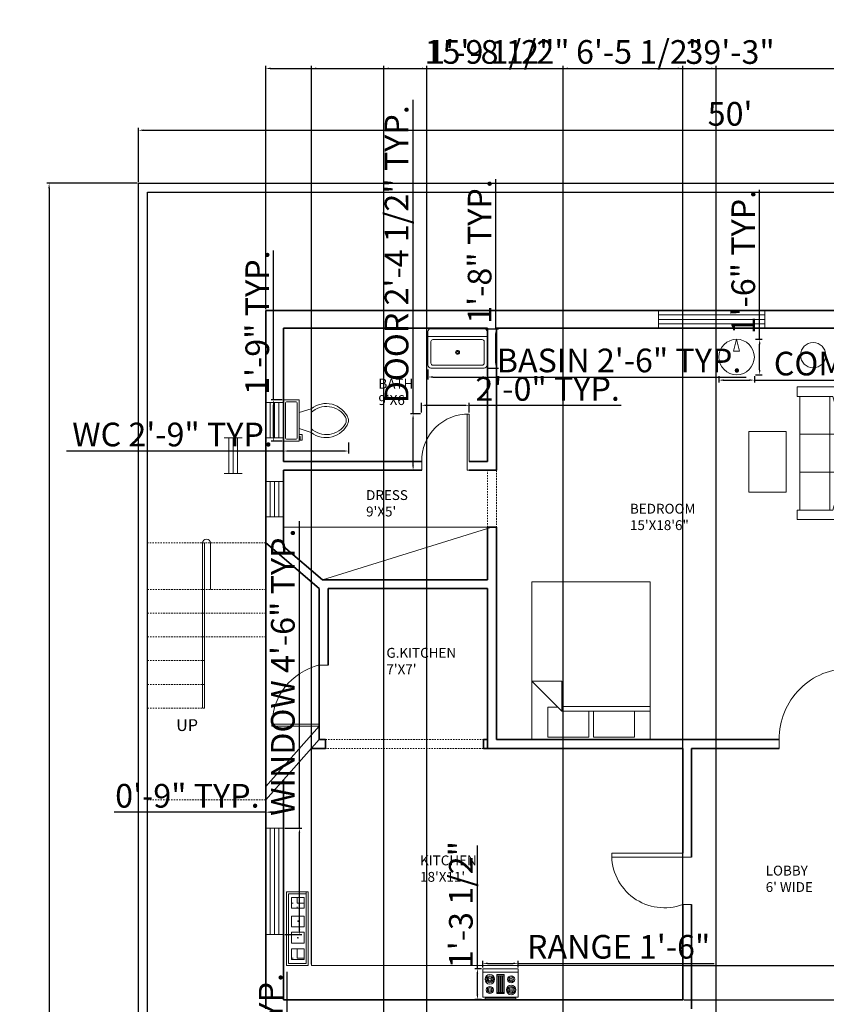
# Model space of a CAD drawing. Units: inches. Extents: x 2562 to 3392, y 1021 to 2243.
# Tile 3 of 6: x 2577 to 2986, y 1744 to 2243. Entities that reach past the tile are written whole.
import ezdxf

# ---------------------------------------------------------------- set-up
doc = ezdxf.new("R2010")
doc.units = ezdxf.units.IN
doc.linetypes.add('JIS_02_0.7', pattern=[1.35, 0.75, -0.6])
for name, color, linetype, lineweight in [('A-ANNO-DIMS', 2, 'Continuous', 18), ('A-ANNO-TEXT', 7, 'Continuous', 18), ('A-AREA-IDEN', 7, 'Continuous', 18), ('A-DOOR', 4, 'Continuous', 18), ('A-EQPM', 9, 'Continuous', 18), ('A-FLOR-CASE', 8, 'Continuous', 18), ('A-FLOR-FIXT', 8, 'Continuous', 18), ('A-FLOR-FIXT-PATT', 252, 'Continuous', 13), ('A-FLOR-STRS', 7, 'Continuous', 18), ('A-FLOR-STRS-HIDN', 8, 'JIS_02_0.7', 13), ('A-FURN', 8, 'Continuous', 18), ('A-GLAZ', 4, 'Continuous', 13), ('A-WALL', 7, 'Continuous', 35), ('A-WALL-HIDN', 7, 'JIS_02_0.7', 18), ('C-PROP', 7, 'Continuous', 30), ('M-EQPM', 9, 'Continuous', 18)]:
    doc.layers.add(name, color=color, linetype=linetype, lineweight=lineweight)
doc.styles.get("Standard").update_dxf_attribs({"font": 'arial.ttf'})
doc.dimstyles.new('ISO-25', dxfattribs={"dimtxt": 12, "dimasz": 2.5, "dimexe": 1.25, "dimexo": 0.625, "dimtad": 1, "dimdec": 1, "dimlunit": 3, "dimtxsty": 'Standard', "dimcen": 2.5, "dimadec": 0, "dimazin": 0, "dimtfac": 1, "dimtdec": 1, "dimtmove": 0, "dimatfit": 3, "dimfxl": 1, "dimarcsym": 0})

# ---------------------------------------------------------------- blocks, each defined once
blk = doc.blocks.new('Toilet - top')
for p, q in [((9.5, -6), (9.5, -2)), ((-10, -8.5), (-8, -8.5)), ((-10, -9.5), (-10, -8.5)), ((-7, -9.5), (-10, -9.5)), ((-8, -8.5), (-8, -8)), ((-7, -8), (-7, -9.5)), ((-4, -8), (-6, -14)), ((4, -8), (6, -14)), ((4, -14), (-4, -14))]:
    blk.add_line(p, q)
blk.add_lwpolyline([(10.5, -8), (10.5, 0), (-10.5, 0), (-10.5, -8)], close=True)
for points in [[(-9.5, -2), (-9.5, -6)], [(8.5, -1), (-8.5, -1)], [(-8.5, -7), (8.5, -7)]]:
    blk.add_lwpolyline(points)
for centre, radius, start, end in [((-8.62, -1.88), 0.884, 81.8699, 188.1301), ((8.62, -1.88), 0.884, 351.8699, 98.1301), ((-8.62, -6.12), 0.884, 171.8699, 278.1301), ((8.62, -6.12), 0.884, 261.8699, 8.1301), ((3.52, -21.58), 12.17, 141.4691, 247.9714), ((4.2, -21.82), 11.33, 136.3677, 238.9468), ((-3.52, -21.58), 12.17, 292.0284, 38.5307), ((-4.2, -21.82), 11.33, 301.053, 43.6321), ((0, -27.88), 4, 245.7318, 294.2682), ((0, -29), 4, 254.8605, 285.1395)]:
    blk.add_arc(centre, radius, start, end)
blk = doc.blocks.new('Sink-single - 30 in top')
blk.add_line((-15, -3.999996), (15, -3.999996))
for points in [[(-13.5, 0), (13.5, 0)], [(-15, -18.499996), (-15, -1.5)], [(15, -1.5), (15, -18.499996)], [(-13.5, -17.499996), (-13.5, -6.499996)], [(-12.5, -5.499996), (12.5, -5.499996)], [(13.5, -6.499996), (13.5, -17.499996)], [(12.5, -18.499996), (-12.5, -18.499996)], [(13.5, -19.999996), (-13.5, -19.999996)]]:
    blk.add_lwpolyline(points)
for radius in [1, 0.5]:
    blk.add_circle((0, -11.999996), radius)
for centre, radius, start, end in [((-13.5, -1.5), 1.5, 90, 180), ((13.5, -1.5), 1.5, 0, 90), ((-12.5, -6.499996), 1, 90, 180), ((12.5, -6.499996), 1, 0, 90), ((-13.5, -18.499996), 1.5, 180, 270), ((-12.5, -17.499996), 1, 180, 270), ((12.5, -17.499996), 1, 270, 0), ((13.5, -18.499996), 1.5, 270, 0)]:
    blk.add_arc(centre, radius, start, end)
blk = doc.blocks.new('Bed - Queen')
for p, q in [((0, -80.00003), (0, 0)), ((0, 0), (59.99999, 0)), ((59.99999, 0), (59.99999, -80.00003)), ((7.99999, -1.2), (28.79998, -1.2)), ((7.99999, -14.4), (7.99999, -1.2)), ((28.79998, -1.2), (28.79998, -14.4)), ((31.19999, -1.2), (51.99999, -1.2)), ((31.19999, -14.4), (31.19999, -1.2)), ((51.99999, -1.2), (51.99999, -16.4)), ((0, -14.4), (44.8, -14.4)), ((59.99999, -29.6), (44.8, -14.4)), ((44.8, -14.4), (44.8, -29.6)), ((44.8, -16.8), (0, -16.8)), ((51.99999, -16.4), (46.79936, -16.4)), ((44.8, -29.6), (59.99999, -29.6)), ((59.99999, -80.00003), (0, -80.00003))]:
    blk.add_line(p, q)
blk = doc.blocks.new('Range-Oven - 30 in top')
for p, q in [((0, -3), (30, -3)), ((12, -6), (18, -6)), ((13, -20), (13, -6)), ((14, -6), (14, -20)), ((15, -20), (15, -6)), ((16, -6), (16, -20)), ((17, -20), (17, -6)), ((6, -24), (6, -25)), ((8, -25), (8, -24)), ((18, -20), (12, -20)), ((22, -25), (22, -24)), ((24, -24), (24, -25))]:
    blk.add_line(p, q)
for points in [[(0, -24), (0, 0), (30, 0), (30, -24)], [(12, -21), (12, -5), (18, -5), (18, -21)], [(2, -26), (2, -25), (28, -25), (28, -26)]]:
    blk.add_lwpolyline(points, close=True)
for centre, radius in [((6, -9), 4), ((6, -9), 3), ((6, -9), 2), ((6, -9), 1), ((24, -9), 3), ((24, -9), 2), ((24, -9), 1), ((6, -18), 3), ((6, -18), 2), ((24, -18), 4), ((24, -18), 3), ((24, -18), 2), ((6, -18), 1), ((24, -18), 1)]:
    blk.add_circle(centre, radius)
blk = doc.blocks.new('Sofa - Roundback 7 ft.')
for p, q in [((-36.000027, -34), (-36.000027, -11.4696)), ((-12.00002, -32.4421), (-12.00003, -6.5971)), ((11.99997, -32.4421), (11.99998, -6.5971)), ((35.99998, -34), (35.99998, -11.4696)), ((-35.999844, -13.3819), (35.9998, -13.3819)), ((-36.000027, -32.4421), (35.99998, -32.4421))]:
    blk.add_line(p, q)
for points in [[(-36.000027, -34), (-42.000027, -34), (-42.000027, -8)], [(41.99998, -8), (41.99998, -34), (35.99998, -34)]]:
    blk.add_lwpolyline(points)
for centre, radius, start, end in [((0, -114.25), 114.25, 68.43141, 111.5686), ((-0.00001, -127.1968), 121.1968, 72.72033, 107.2797)]:
    blk.add_arc(centre, radius, start, end)
blk = doc.blocks.new('Compressor')
for p, q in [((0, 0), (-0.05, -0.2)), ((0.05, -0.2), (0, 0)), ((-0.05, -0.2), (0.05, -0.2))]:
    blk.add_line(p, q)
blk.add_circle((0, -0.3), 0.3)
blk = doc.blocks.new('Window - Wood Frame 36 in. Wide plan')
for p, q in [((0, 6), (0, 0)), ((0, 4.5), (36, 4.5)), ((36, 6), (36, 0)), ((0, 3), (36, 3)), ((0, 1.5), (36, 1.5))]:
    blk.add_line(p, q)
blk = doc.blocks.new('*D21')
at = {"layer": 'A-ANNO-DIMS', "color": 0, "lineweight": -2, "transparency": 16777216}
for p, q in [((2636.76, 2160.76), (2636.76, 2188.27)), ((2639.26, 2187.02), (3234.26, 2187.02)), ((3236.76, 2160.76), (3236.76, 2188.27))]:
    blk.add_line(p, q, dxfattribs=at)
at = {"layer": 'A-ANNO-DIMS', "color": 0, "transparency": 16777216}
for points in [[(2639.26, 2187.43), (2639.26, 2186.6), (2636.76, 2187.02)], [(3234.26, 2187.43), (3234.26, 2186.6), (3236.76, 2187.02)]]:
    blk.add_solid(points, dxfattribs=at)
at = {"layer": 'Defpoints', "color": 0, "transparency": 16777216}
for p in [(3236.76, 2187.02), (2636.76, 2160.13), (3236.76, 2160.13)]:
    blk.add_point(p, dxfattribs=at)
at = {"layer": 'A-ANNO-DIMS', "color": 0, "transparency": 16777216, "insert": (2936.76, 2193.77), "char_height": 12, "attachment_point": 5}
blk.add_mtext("50'", dxfattribs=at)
blk = doc.blocks.new('*D22')
at = {"layer": 'A-ANNO-DIMS', "color": 0, "lineweight": -2, "transparency": 16777216}
for p, q in [((2636.14, 2160.13), (2590.2, 2160.13)), ((2591.45, 2157.63), (2591.45, 1082.63)), ((2636.14, 1080.13), (2590.2, 1080.13))]:
    blk.add_line(p, q, dxfattribs=at)
at = {"layer": 'A-ANNO-DIMS', "color": 0, "transparency": 16777216}
for points in [[(2591.03, 2157.63), (2591.86, 2157.63), (2591.45, 2160.13)], [(2591.03, 1082.63), (2591.86, 1082.63), (2591.45, 1080.13)]]:
    blk.add_solid(points, dxfattribs=at)
at = {"layer": 'Defpoints', "color": 0, "transparency": 16777216}
for p in [(2636.76, 2160.13), (2591.45, 1080.13), (2636.76, 1080.13)]:
    blk.add_point(p, dxfattribs=at)
at = {"layer": 'A-ANNO-DIMS', "color": 0, "transparency": 16777216, "insert": (2584.7, 1620.13), "char_height": 12, "attachment_point": 5, "rotation": 90}
blk.add_mtext("90'", dxfattribs=at)
blk = doc.blocks.new('DOOR-SWING-24IN')
for p, q in [((24.01, 28.5), (23.01, 28.5)), ((23.01, 28.5), (23.01, 0)), ((24.01, 4.5), (24.01, 28.5)), ((0.01, 4.5), (0.01, 0))]:
    blk.add_line(p, q)
blk.add_arc((23.51, 5), 23.51, 88.7811, 181.2189)
blk = doc.blocks.new('*D25')
at = {"layer": 'A-ANNO-DIMS', "color": 0, "lineweight": -2, "transparency": 16777216}
for p, q in [((2718.36, 1833.2), (2718.36, 1988.8)), ((2710.89, 1833.2), (2719.61, 1833.2)), ((2718.36, 1781.7), (2718.36, 1830.7)), ((2710.89, 1779.2), (2719.61, 1779.2))]:
    blk.add_line(p, q, dxfattribs=at)
at = {"layer": 'A-ANNO-DIMS', "color": 0, "transparency": 16777216}
for points in [[(2717.95, 1830.7), (2718.78, 1830.7), (2718.36, 1833.2)], [(2717.95, 1781.7), (2718.78, 1781.7), (2718.36, 1779.2)]]:
    blk.add_solid(points, dxfattribs=at)
at = {"layer": 'Defpoints', "color": 0, "transparency": 16777216}
for p in [(2710.26, 1833.2), (2718.36, 1833.2), (2710.26, 1779.2)]:
    blk.add_point(p, dxfattribs=at)
at = {"layer": 'A-ANNO-DIMS', "color": 0, "transparency": 16777216, "insert": (2711.53, 1912.25), "char_height": 12, "attachment_point": 5, "rotation": 90}
blk.add_mtext('WINDOW 4\'-6" TYP.', dxfattribs=at)
blk = doc.blocks.new('*D26')
at = {"layer": 'A-ANNO-DIMS', "color": 0, "lineweight": -2, "transparency": 16777216}
for p, q in [((2701.26, 1833.83), (2701.26, 1842.55)), ((2710.26, 1833.83), (2710.26, 1842.55)), ((2701.26, 1841.3), (2624.37, 1841.3)), ((2707.76, 1841.3), (2703.76, 1841.3))]:
    blk.add_line(p, q, dxfattribs=at)
at = {"layer": 'A-ANNO-DIMS', "color": 0, "transparency": 16777216}
for points in [[(2703.76, 1841.72), (2703.76, 1840.88), (2701.26, 1841.3)], [(2707.76, 1841.72), (2707.76, 1840.88), (2710.26, 1841.3)]]:
    blk.add_solid(points, dxfattribs=at)
at = {"layer": 'Defpoints', "color": 0, "transparency": 16777216}
for p in [(2701.26, 1841.3), (2701.26, 1833.2), (2710.26, 1833.2)]:
    blk.add_point(p, dxfattribs=at)
at = {"layer": 'A-ANNO-DIMS', "color": 0, "transparency": 16777216, "insert": (2661.56, 1848.05), "char_height": 12, "attachment_point": 5}
blk.add_mtext('0\'-9" TYP.', dxfattribs=at)
blk = doc.blocks.new('*D31')
at = {"layer": 'A-ANNO-DIMS', "color": 0, "lineweight": -2, "transparency": 16777216}
for p, q in [((2776.02, 2043.27), (2776.02, 2202.48)), ((2779.69, 2043.27), (2774.77, 2043.27)), ((2776.02, 2017.13), (2776.02, 2040.77)), ((2779.69, 2014.63), (2774.77, 2014.63))]:
    blk.add_line(p, q, dxfattribs=at)
at = {"layer": 'A-ANNO-DIMS', "color": 0, "transparency": 16777216}
for points in [[(2775.6, 2040.77), (2776.43, 2040.77), (2776.02, 2043.27)], [(2775.6, 2017.13), (2776.43, 2017.13), (2776.02, 2014.63)]]:
    blk.add_solid(points, dxfattribs=at)
at = {"layer": 'Defpoints', "color": 0, "transparency": 16777216}
for p in [(2776.02, 2043.27), (2780.31, 2043.27), (2780.31, 2014.63)]:
    blk.add_point(p, dxfattribs=at)
at = {"layer": 'A-ANNO-DIMS', "color": 0, "transparency": 16777216, "insert": (2769.18, 2124.12), "char_height": 12, "attachment_point": 5, "rotation": 90}
blk.add_mtext('DOOR 2\'-4 1/2" TYP.', dxfattribs=at)
blk = doc.blocks.new('*D32')
at = {"layer": 'A-ANNO-DIMS', "color": 0, "lineweight": -2, "transparency": 16777216}
for p, q in [((2780.31, 2043.89), (2780.31, 2048.81)), ((2782.81, 2047.56), (2801.95, 2047.56)), ((2804.45, 2043.89), (2804.45, 2048.81)), ((2804.45, 2047.56), (2881.55, 2047.56))]:
    blk.add_line(p, q, dxfattribs=at)
at = {"layer": 'A-ANNO-DIMS', "color": 0, "transparency": 16777216}
for points in [[(2782.81, 2047.98), (2782.81, 2047.15), (2780.31, 2047.56)], [(2801.95, 2047.98), (2801.95, 2047.15), (2804.45, 2047.56)]]:
    blk.add_solid(points, dxfattribs=at)
at = {"layer": 'Defpoints', "color": 0, "transparency": 16777216}
for p in [(2804.45, 2047.56), (2780.31, 2043.27), (2804.45, 2043.27)]:
    blk.add_point(p, dxfattribs=at)
at = {"layer": 'A-ANNO-DIMS', "color": 0, "transparency": 16777216, "insert": (2844.25, 2054.32), "char_height": 12, "attachment_point": 5}
blk.add_mtext('2\'-0" TYP.', dxfattribs=at)
blk = doc.blocks.new('*D35')
at = {"layer": 'A-ANNO-DIMS', "color": 0, "lineweight": -2, "transparency": 16777216}
for p, q in [((2710.26, 2028.71), (2710.26, 2023.13)), ((2743.31, 2028.71), (2743.31, 2023.13)), ((2710.26, 2024.38), (2600.29, 2024.38)), ((2740.81, 2024.38), (2712.76, 2024.38))]:
    blk.add_line(p, q, dxfattribs=at)
at = {"layer": 'A-ANNO-DIMS', "color": 0, "transparency": 16777216}
for points in [[(2712.76, 2024.79), (2712.76, 2023.96), (2710.26, 2024.38)], [(2740.81, 2024.79), (2740.81, 2023.96), (2743.31, 2024.38)]]:
    blk.add_solid(points, dxfattribs=at)
at = {"layer": 'Defpoints', "color": 0, "transparency": 16777216}
for p in [(2710.26, 2029.33), (2743.31, 2029.33), (2710.26, 2024.38)]:
    blk.add_point(p, dxfattribs=at)
at = {"layer": 'A-ANNO-DIMS', "color": 0, "transparency": 16777216, "insert": (2654.03, 2031.21), "char_height": 12, "attachment_point": 5}
blk.add_mtext('WC 2\'-9" TYP.', dxfattribs=at)
blk = doc.blocks.new('*D36')
at = {"layer": 'A-ANNO-DIMS', "color": 0, "lineweight": -2, "transparency": 16777216}
for p, q in [((2705.31, 2050.33), (2705.31, 2126.1)), ((2709.64, 2050.33), (2704.06, 2050.33)), ((2705.31, 2031.83), (2705.31, 2047.83)), ((2709.64, 2029.33), (2704.06, 2029.33))]:
    blk.add_line(p, q, dxfattribs=at)
at = {"layer": 'A-ANNO-DIMS', "color": 0, "transparency": 16777216}
for points in [[(2704.89, 2047.83), (2705.72, 2047.83), (2705.31, 2050.33)], [(2704.89, 2031.83), (2705.72, 2031.83), (2705.31, 2029.33)]]:
    blk.add_solid(points, dxfattribs=at)
at = {"layer": 'Defpoints', "color": 0, "transparency": 16777216}
for p in [(2705.31, 2050.33), (2710.26, 2050.33), (2710.26, 2029.33)]:
    blk.add_point(p, dxfattribs=at)
at = {"layer": 'A-ANNO-DIMS', "color": 0, "transparency": 16777216, "insert": (2698.55, 2089.47), "char_height": 12, "attachment_point": 5, "rotation": 90}
blk.add_mtext('1\'-9" TYP.', dxfattribs=at)
blk = doc.blocks.new('*D37')
at = {"layer": 'A-ANNO-DIMS', "color": 0, "lineweight": -2, "transparency": 16777216}
for p, q in [((2783.55, 2065.78), (2783.55, 2060.66)), ((2786.05, 2061.91), (2811.05, 2061.91)), ((2813.55, 2065.78), (2813.55, 2060.66)), ((2813.55, 2061.91), (2944.88, 2061.91))]:
    blk.add_line(p, q, dxfattribs=at)
at = {"layer": 'A-ANNO-DIMS', "color": 0, "transparency": 16777216}
for points in [[(2786.05, 2062.32), (2786.05, 2061.49), (2783.55, 2061.91)], [(2811.05, 2062.32), (2811.05, 2061.49), (2813.55, 2061.91)]]:
    blk.add_solid(points, dxfattribs=at)
at = {"layer": 'Defpoints', "color": 0, "transparency": 16777216}
for p in [(2783.55, 2066.41), (2813.55, 2066.41), (2813.55, 2061.91)]:
    blk.add_point(p, dxfattribs=at)
at = {"layer": 'A-ANNO-DIMS', "color": 0, "transparency": 16777216, "insert": (2880.46, 2068.74), "char_height": 12, "attachment_point": 5}
blk.add_mtext('BASIN 2\'-6" TYP.', dxfattribs=at)
blk = doc.blocks.new('*D38')
at = {"layer": 'A-ANNO-DIMS', "color": 0, "lineweight": -2, "transparency": 16777216}
for p, q in [((2818.05, 2086.41), (2818.05, 2162.17)), ((2814.17, 2086.41), (2819.3, 2086.41)), ((2818.05, 2068.91), (2818.05, 2083.91)), ((2814.17, 2066.41), (2819.3, 2066.41))]:
    blk.add_line(p, q, dxfattribs=at)
at = {"layer": 'A-ANNO-DIMS', "color": 0, "transparency": 16777216}
for points in [[(2817.63, 2083.91), (2818.47, 2083.91), (2818.05, 2086.41)], [(2817.63, 2068.91), (2818.47, 2068.91), (2818.05, 2066.41)]]:
    blk.add_solid(points, dxfattribs=at)
at = {"layer": 'Defpoints', "color": 0, "transparency": 16777216}
for p in [(2813.55, 2086.41), (2818.05, 2086.41), (2813.55, 2066.41)]:
    blk.add_point(p, dxfattribs=at)
at = {"layer": 'A-ANNO-DIMS', "color": 0, "transparency": 16777216, "insert": (2811.3, 2125.54), "char_height": 12, "attachment_point": 5, "rotation": 90}
blk.add_mtext('1\'-8" TYP.', dxfattribs=at)
blk = doc.blocks.new('*D41')
at = {"layer": 'A-ANNO-DIMS', "color": 0, "lineweight": -2, "transparency": 16777216}
for p, q in [((2931.06, 2062.4), (2931.06, 2059.08)), ((2949.06, 2062.4), (2949.06, 2059.08)), ((2933.56, 2060.33), (2946.56, 2060.33)), ((2949.06, 2060.33), (3151.56, 2060.33))]:
    blk.add_line(p, q, dxfattribs=at)
at = {"layer": 'A-ANNO-DIMS', "color": 0, "transparency": 16777216}
for points in [[(2933.56, 2060.75), (2933.56, 2059.91), (2931.06, 2060.33)], [(2946.56, 2060.75), (2946.56, 2059.91), (2949.06, 2060.33)]]:
    blk.add_solid(points, dxfattribs=at)
at = {"layer": 'Defpoints', "color": 0, "transparency": 16777216}
for p in [(2931.06, 2063.03), (2949.06, 2063.03), (2949.06, 2060.33)]:
    blk.add_point(p, dxfattribs=at)
at = {"layer": 'A-ANNO-DIMS', "color": 0, "transparency": 16777216, "insert": (3051.56, 2067.16), "char_height": 12, "attachment_point": 5}
blk.add_mtext('COMPRESSOR 1\'-6" TYP.', dxfattribs=at)
blk = doc.blocks.new('*D42')
at = {"layer": 'A-ANNO-DIMS', "color": 0, "lineweight": -2, "transparency": 16777216}
for p, q in [((2951.76, 2081.03), (2951.76, 2156.79)), ((2949.68, 2081.03), (2953.01, 2081.03)), ((2951.76, 2065.53), (2951.76, 2078.53)), ((2949.68, 2063.03), (2953.01, 2063.03))]:
    blk.add_line(p, q, dxfattribs=at)
at = {"layer": 'A-ANNO-DIMS', "color": 0, "transparency": 16777216}
for points in [[(2951.34, 2078.53), (2952.18, 2078.53), (2951.76, 2081.03)], [(2951.34, 2065.53), (2952.18, 2065.53), (2951.76, 2063.03)]]:
    blk.add_solid(points, dxfattribs=at)
at = {"layer": 'Defpoints', "color": 0, "transparency": 16777216}
for p in [(2949.06, 2081.03), (2951.76, 2081.03), (2949.06, 2063.03)]:
    blk.add_point(p, dxfattribs=at)
at = {"layer": 'A-ANNO-DIMS', "color": 0, "transparency": 16777216, "insert": (2945.01, 2120.16), "char_height": 12, "attachment_point": 5, "rotation": 90}
blk.add_mtext('1\'-6" TYP.', dxfattribs=at)
blk = doc.blocks.new('*D45')
at = {"layer": 'A-ANNO-DIMS', "color": 0, "lineweight": -2, "transparency": 16777216}
for p, q in [((2811.33, 1762.57), (2811.33, 1765.9)), ((2813.83, 1764.65), (2826.83, 1764.65)), ((2829.33, 1762.57), (2829.33, 1765.9)), ((2829.33, 1764.65), (2928.63, 1764.65))]:
    blk.add_line(p, q, dxfattribs=at)
at = {"layer": 'A-ANNO-DIMS', "color": 0, "transparency": 16777216}
for points in [[(2813.83, 1765.06), (2813.83, 1764.23), (2811.33, 1764.65)], [(2826.83, 1765.06), (2826.83, 1764.23), (2829.33, 1764.65)]]:
    blk.add_solid(points, dxfattribs=at)
at = {"layer": 'Defpoints', "color": 0, "transparency": 16777216}
for p in [(2829.33, 1764.65), (2811.33, 1761.95), (2829.33, 1761.95)]:
    blk.add_point(p, dxfattribs=at)
at = {"layer": 'A-ANNO-DIMS', "color": 0, "transparency": 16777216, "insert": (2880.23, 1771.48), "char_height": 12, "attachment_point": 5}
blk.add_mtext('RANGE 1\'-6"', dxfattribs=at)
blk = doc.blocks.new('*D46')
at = {"layer": 'A-ANNO-DIMS', "color": 0, "lineweight": -2, "transparency": 16777216}
for p, q in [((2808.63, 1761.95), (2808.63, 1824.43)), ((2810.7, 1761.95), (2807.38, 1761.95)), ((2808.63, 1748.85), (2808.63, 1759.45)), ((2810.7, 1746.35), (2807.38, 1746.35))]:
    blk.add_line(p, q, dxfattribs=at)
at = {"layer": 'A-ANNO-DIMS', "color": 0, "transparency": 16777216}
for points in [[(2808.21, 1759.45), (2809.04, 1759.45), (2808.63, 1761.95)], [(2808.21, 1748.85), (2809.04, 1748.85), (2808.63, 1746.35)]]:
    blk.add_solid(points, dxfattribs=at)
at = {"layer": 'Defpoints', "color": 0, "transparency": 16777216}
for p in [(2808.63, 1761.95), (2811.33, 1761.95), (2811.33, 1746.35)]:
    blk.add_point(p, dxfattribs=at)
at = {"layer": 'A-ANNO-DIMS', "color": 0, "transparency": 16777216, "insert": (2801.79, 1794.44), "char_height": 12, "attachment_point": 5, "rotation": 90}
blk.add_mtext('1\'-3 1/2"', dxfattribs=at)
blk = doc.blocks.new('*D66')
at = {"layer": 'A-ANNO-DIMS', "color": 0, "lineweight": -2, "transparency": 16777216}
for p, q in [((2712.12, 1683.33), (2712.12, 1760.43)), ((2717.11, 1683.33), (2710.87, 1683.33)), ((2712.12, 1655.66), (2712.12, 1680.83)), ((2717.11, 1653.16), (2710.87, 1653.16))]:
    blk.add_line(p, q, dxfattribs=at)
at = {"layer": 'A-ANNO-DIMS', "color": 0, "transparency": 16777216}
for points in [[(2711.71, 1680.83), (2712.54, 1680.83), (2712.12, 1683.33)], [(2711.71, 1655.66), (2712.54, 1655.66), (2712.12, 1653.16)]]:
    blk.add_solid(points, dxfattribs=at)
at = {"layer": 'Defpoints', "color": 0, "transparency": 16777216}
for p in [(2712.12, 1683.33), (2717.73, 1683.33), (2717.73, 1653.16)]:
    blk.add_point(p, dxfattribs=at)
at = {"layer": 'A-ANNO-DIMS', "color": 0, "transparency": 16777216, "insert": (2705.37, 1723.13), "char_height": 12, "attachment_point": 5, "rotation": 90}
blk.add_mtext('2\'-6" TYP.', dxfattribs=at)
blk = doc.blocks.new('*D69')
at = {"layer": 'A-ANNO-DIMS', "color": 0, "lineweight": -2, "transparency": 16777216}
for p, q in [((2701.26, 2096.26), (2701.26, 2219.58)), ((2703.76, 2218.33), (3169.76, 2218.33)), ((3172.26, 2096.26), (3172.26, 2219.58))]:
    blk.add_line(p, q, dxfattribs=at)
at = {"layer": 'A-ANNO-DIMS', "color": 0, "transparency": 16777216}
for points in [[(2703.76, 2218.75), (2703.76, 2217.92), (2701.26, 2218.33)], [(3169.76, 2218.75), (3169.76, 2217.92), (3172.26, 2218.33)]]:
    blk.add_solid(points, dxfattribs=at)
at = {"layer": 'Defpoints', "color": 0, "transparency": 16777216}
for p in [(3172.26, 2218.33), (2701.26, 2095.63), (3172.26, 2095.63)]:
    blk.add_point(p, dxfattribs=at)
at = {"layer": 'A-ANNO-DIMS', "color": 0, "transparency": 16777216, "insert": (2936.76, 2225.09), "char_height": 12, "attachment_point": 5}
blk.add_mtext('39\'-3"', dxfattribs=at)
blk = doc.blocks.new('*D74')
at = {"layer": 'A-ANNO-DIMS', "color": 0, "lineweight": -2, "transparency": 16777216}
for p, q in [((2852.07, 1483.26), (2852.07, 2219.58)), ((2854.57, 2218.33), (2927.14, 2218.33)), ((2929.64, 1483.26), (2929.64, 2219.58))]:
    blk.add_line(p, q, dxfattribs=at)
at = {"layer": 'A-ANNO-DIMS', "color": 0, "transparency": 16777216}
for points in [[(2854.57, 2218.75), (2854.57, 2217.92), (2852.07, 2218.33)], [(2927.14, 2218.75), (2927.14, 2217.92), (2929.64, 2218.33)]]:
    blk.add_solid(points, dxfattribs=at)
at = {"layer": 'Defpoints', "color": 0, "transparency": 16777216}
for p in [(2929.64, 2218.33), (2852.07, 1482.63), (2929.64, 1482.63)]:
    blk.add_point(p, dxfattribs=at)
at = {"layer": 'A-ANNO-DIMS', "color": 0, "transparency": 16777216, "insert": (2890.85, 2225.16), "char_height": 12, "attachment_point": 5}
blk.add_mtext('6\'-5 1/2"', dxfattribs=at)
blk = doc.blocks.new('*D75')
at = {"layer": 'A-ANNO-DIMS', "color": 0, "lineweight": -2, "transparency": 16777216}
for p, q in [((2724.45, 1764.19), (2724.45, 2219.58)), ((2726.95, 2218.33), (2910.26, 2218.33)), ((2912.76, 1764.19), (2912.76, 2219.58))]:
    blk.add_line(p, q, dxfattribs=at)
at = {"layer": 'A-ANNO-DIMS', "color": 0, "transparency": 16777216}
for points in [[(2726.95, 2218.75), (2726.95, 2217.92), (2724.45, 2218.33)], [(2910.26, 2218.75), (2910.26, 2217.92), (2912.76, 2218.33)]]:
    blk.add_solid(points, dxfattribs=at)
at = {"layer": 'Defpoints', "color": 0, "transparency": 16777216}
for p in [(2912.76, 2218.33), (2724.45, 1763.57), (2912.76, 1763.57)]:
    blk.add_point(p, dxfattribs=at)
at = {"layer": 'A-ANNO-DIMS', "color": 0, "transparency": 16777216, "insert": (2818.6, 2225.16), "char_height": 12, "attachment_point": 5}
blk.add_mtext('15\'-8 1/2"', dxfattribs=at)
blk = doc.blocks.new('*D76')
at = {"layer": 'A-ANNO-DIMS', "color": 0, "lineweight": -2, "transparency": 16777216}
for p, q in [((3294.96, 1763.57), (3294.96, 1826.05)), ((2913.39, 1763.57), (3296.21, 1763.57)), ((3294.96, 1748.63), (3294.96, 1761.07)), ((2913.39, 1746.13), (3296.21, 1746.13))]:
    blk.add_line(p, q, dxfattribs=at)
at = {"layer": 'A-ANNO-DIMS', "color": 0, "transparency": 16777216}
for points in [[(3294.55, 1761.07), (3295.38, 1761.07), (3294.96, 1763.57)], [(3294.55, 1748.63), (3295.38, 1748.63), (3294.96, 1746.13)]]:
    blk.add_solid(points, dxfattribs=at)
at = {"layer": 'Defpoints', "color": 0, "transparency": 16777216}
for p in [(2912.76, 1763.57), (3294.96, 1763.57), (2912.76, 1746.13)]:
    blk.add_point(p, dxfattribs=at)
at = {"layer": 'A-ANNO-DIMS', "color": 0, "transparency": 16777216, "insert": (3288.13, 1796.06), "char_height": 12, "attachment_point": 5, "rotation": 90}
blk.add_mtext('1\'-5 1/2"', dxfattribs=at)
blk = doc.blocks.new('*D79')
at = {"layer": 'A-ANNO-DIMS', "color": 0, "lineweight": -2, "transparency": 16777216}
for p, q in [((2761.26, 1555.09), (2761.26, 2219.58)), ((2763.76, 2218.33), (2780.46, 2218.33)), ((2782.96, 1555.09), (2782.96, 2219.58)), ((2782.96, 2218.33), (2845.44, 2218.33))]:
    blk.add_line(p, q, dxfattribs=at)
at = {"layer": 'A-ANNO-DIMS', "color": 0, "transparency": 16777216}
for points in [[(2763.76, 2218.75), (2763.76, 2217.92), (2761.26, 2218.33)], [(2780.46, 2218.75), (2780.46, 2217.92), (2782.96, 2218.33)]]:
    blk.add_solid(points, dxfattribs=at)
at = {"layer": 'Defpoints', "color": 0, "transparency": 16777216}
for p in [(2782.96, 2218.33), (2761.26, 1554.47), (2782.96, 1554.47)]:
    blk.add_point(p, dxfattribs=at)
at = {"layer": 'A-ANNO-DIMS', "color": 0, "transparency": 16777216, "insert": (2815.45, 2225.16), "char_height": 12, "attachment_point": 5}
blk.add_mtext('1\'-9 1/2"', dxfattribs=at)

msp = doc.modelspace()

# ---------------------------------------------------------------- hatches: boundary and pattern name
at = {"layer": 'A-FLOR-FIXT-PATT'}
h = msp.add_hatch(dxfattribs=at)
h.set_pattern_fill('ANGLE', color=256)
h.set_pattern_definition([(0, (0, 0), (0, 6.985), [5.08, -1.905]), (90, (0, 0), (-6.985, 4e-16), [5.08, -1.905])])
h.paths.add_polyline_path([(2720.79, 1798.07), (2714.4, 1798.07), (2714.4, 1792.54), (2720.79, 1792.54)])
h.paths.add_polyline_path([(2720.74, 1772.07), (2714.34, 1772.07), (2714.34, 1766.54), (2720.74, 1766.54)])

# ---------------------------------------------------------------- linework, layer by layer
at = {"layer": 'A-DOOR'}
for p, q in [((2803.45, 2014.63), (2804.45, 2014.63)), ((2732.94, 1915.78), (2728.44, 1915.78)), ((2704.44, 1884.91), (2704.44, 1885.91)), ((2704.44, 1885.91), (2728.44, 1885.91)), ((2728.44, 1884.91), (2704.44, 1884.91)), ((2961.71, 1878.13), (2961.71, 1873.63)), ((2912.76, 1820.5), (2876.76, 1820.5)), ((2876.76, 1820.5), (2876.76, 1818.5)), ((2876.76, 1818.5), (2917.26, 1818.5)), ((2912.76, 1794.5), (2917.26, 1794.5))]:
    msp.add_line(p, q, dxfattribs=at)
for centre, radius, start, end in [((2735.81, 1885.41), 31.38, 103.5921, 180.913), ((2997.21, 1878.63), 35.5, 89.1931, 180.8069), ((2903.43, 1819.5), 26.69, 177.8524, 290.4723)]:
    msp.add_arc(centre, radius, start, end, dxfattribs=at)
at = {"layer": 'A-FLOR-CASE'}
for p, q in [((2816.01, 1985.77), (2710.26, 1985.77)), ((2730.09, 1959.13), (2816.01, 1985.77)), ((2724.45, 1873.63), (2724.45, 1763.57)), ((2724.45, 1763.57), (2912.76, 1763.57))]:
    msp.add_line(p, q, dxfattribs=at)
at = {"layer": 'A-FLOR-FIXT'}
for p, q in [((2711.87, 1800.82), (2711.87, 1763.57)), ((2722.74, 1800.82), (2711.87, 1800.82)), ((2721.74, 1799.82), (2712.87, 1799.82)), ((2712.87, 1799.82), (2712.87, 1764.57)), ((2721.74, 1764.57), (2721.74, 1800.82)), ((2722.74, 1763.57), (2722.74, 1800.82)), ((2711.87, 1763.57), (2722.74, 1763.57)), ((2712.87, 1764.57), (2721.74, 1764.57))]:
    msp.add_line(p, q, dxfattribs=at)
for points in [[(2714.4, 1798.07), (2720.79, 1798.07), (2720.79, 1792.54), (2714.4, 1792.54)], [(2714.34, 1788.61), (2720.74, 1788.61), (2720.74, 1783.08), (2714.34, 1783.08)], [(2714.34, 1780.39), (2720.74, 1780.39), (2720.74, 1774.86), (2714.34, 1774.86)], [(2714.34, 1772.07), (2720.74, 1772.07), (2720.74, 1766.54), (2714.34, 1766.54)]]:
    msp.add_lwpolyline(points, close=True, dxfattribs=at)
for centre in [(2717.71, 1786.02), (2717.54, 1777.63)]:
    msp.add_circle(centre, 0.174, dxfattribs=at)
at = {"layer": 'A-FLOR-STRS'}
for p, q in [((2669.26, 1977.76), (2669.26, 1894.1)), ((2670.26, 1977.76), (2670.26, 1894.1)), ((2673.26, 1977.76), (2673.26, 1954.1))]:
    msp.add_line(p, q, dxfattribs=at)
msp.add_arc((2671.26, 1977.76), 2, 0, 180, dxfattribs=at)
at = {"layer": 'A-FLOR-STRS-HIDN'}
for p, q in [((2701.26, 1977.76), (2641.26, 1977.76)), ((2641.26, 1954.1), (2701.26, 1954.1)), ((2641.26, 1942.1), (2701.26, 1942.1)), ((2641.26, 1930.1), (2701.26, 1930.1)), ((2641.26, 1918.1), (2670.26, 1918.1)), ((2641.26, 1906.1), (2670.26, 1906.1)), ((2641.26, 1894.1), (2670.26, 1894.1)), ((2701.26, 1847.5), (2641.26, 1847.5))]:
    msp.add_line(p, q, dxfattribs=at)
at = {"layer": 'A-FURN'}
msp.add_lwpolyline([(2946.23, 2034.23), (2965.12, 2034.23), (2965.12, 2003.47), (2946.23, 2003.47)], close=True, dxfattribs=at)
msp.add_circle((2978.9, 2072.96), 6.38, dxfattribs=at)
at = {"layer": 'A-WALL'}
for p, q in [((2701.26, 2095.63), (3172.26, 2095.63)), ((2701.26, 1741.63), (2701.26, 2095.63)), ((2710.26, 2086.63), (2813.76, 2086.63)), ((2710.26, 2019.13), (2710.26, 2086.63)), ((2813.76, 2019.13), (2813.76, 2086.63)), ((2818.26, 2086.63), (3007.26, 2086.63)), ((2818.26, 2014.63), (2818.26, 2086.63)), ((2710.26, 2019.13), (2780.45, 2019.13)), ((2804.45, 2019.13), (2813.76, 2019.13)), ((2710.26, 2014.63), (2780.45, 2014.63)), ((2710.26, 1976.01), (2710.26, 2014.63)), ((2804.45, 2014.63), (2813.76, 2014.63)), ((2813.76, 2014.63), (2818.26, 2014.63)), ((2813.76, 1959.13), (2813.76, 1985.77)), ((2813.76, 1985.77), (2818.26, 1985.77)), ((2818.26, 1878.13), (2818.26, 1985.77)), ((2701.26, 1977.76), (2728.44, 1954.63)), ((2710.26, 1976.01), (2730.09, 1959.13)), ((2730.09, 1959.13), (2813.76, 1959.13)), ((2728.44, 1954.63), (2728.44, 1930.63)), ((2732.94, 1954.63), (2813.76, 1954.63)), ((2732.94, 1930.63), (2732.94, 1954.63)), ((2813.76, 1873.63), (2813.76, 1954.63)), ((2728.44, 1930.63), (2728.44, 1878.13)), ((2732.94, 1930.63), (2732.94, 1915.78)), ((2728.44, 1884.91), (2701.26, 1854.28)), ((2728.44, 1878.13), (2701.26, 1847.5)), ((2728.44, 1878.13), (2731.53, 1878.13)), ((2731.53, 1878.13), (2731.53, 1873.63)), ((2811.67, 1878.13), (2811.67, 1873.63)), ((2811.67, 1878.13), (2813.76, 1878.13)), ((2818.26, 1878.13), (2961.71, 1878.13)), ((2724.45, 1873.63), (2731.53, 1873.63)), ((2811.67, 1873.63), (2912.76, 1873.63)), ((2912.76, 1820.5), (2912.76, 1873.63)), ((2917.26, 1818.5), (2917.26, 1873.63)), ((2917.26, 1873.63), (2961.71, 1873.63)), ((2710.26, 1746.13), (2710.26, 1857.64)), ((2912.76, 1746.13), (2912.76, 1794.5)), ((2917.26, 1741.63), (2917.26, 1794.5)), ((2710.26, 1746.13), (2912.76, 1746.13))]:
    msp.add_line(p, q, dxfattribs=at)
at = {"layer": 'A-WALL-HIDN'}
for p, q in [((2813.76, 1985.77), (2813.76, 2014.63)), ((2818.26, 2014.63), (2818.26, 1985.77)), ((2731.53, 1878.13), (2811.67, 1878.13)), ((2811.67, 1873.63), (2731.53, 1873.63))]:
    msp.add_line(p, q, dxfattribs=at)
at = {"layer": 'C-PROP'}
for p, q in [((2636.76, 2160.13), (3236.76, 2160.13)), ((2636.76, 1080.13), (2636.76, 2160.13)), ((2641.26, 2155.63), (3232.26, 2155.63)), ((2641.26, 1084.63), (2641.26, 2155.63))]:
    msp.add_line(p, q, dxfattribs=at)

# ---------------------------------------------------------------- block references
at = {"layer": 'A-DOOR'}
msp.add_blockref('DOOR-SWING-24IN', (2780.44, 2014.63), dxfattribs=at)
at = {"layer": 'A-EQPM', "xscale": 0.6, "yscale": 0.6}
msp.add_blockref('Range-Oven - 30 in top', (2811.33, 1761.95), dxfattribs=at)
at = {"layer": 'A-FLOR-FIXT'}
msp.add_blockref('Sink-single - 30 in top', (2798.55, 2086.41), dxfattribs=at)
at = {"layer": 'A-FLOR-FIXT', "rotation": 90}
msp.add_blockref('Toilet - top', (2710.26, 2039.83), dxfattribs=at)
at = {"layer": 'A-FURN', "xscale": 0.8, "yscale": 0.8, "rotation": 270}
msp.add_blockref('Sofa - Roundback 7 ft.', (2998.06, 2023.25), dxfattribs=at)
at = {"layer": 'A-FURN', "rotation": 180}
msp.add_blockref('Bed - Queen', (2896.26, 1878.13), dxfattribs=at)
at = {"layer": 'A-GLAZ', "xscale": 1.5, "yscale": 1.5}
msp.add_blockref('Window - Wood Frame 36 in. Wide plan', (2900.38, 2086.63), dxfattribs=at)
at = {"layer": 'A-GLAZ', "yscale": 1.5, "rotation": 90}
for p, xscale in [((2710.26, 2031.04), 0.5), ((2689.26, 2013.04), 0.5), ((2710.26, 1990.95), 0.5), ((2710.26, 1779.2), 1.5)]:
    msp.add_blockref('Window - Wood Frame 36 in. Wide plan', p, dxfattribs=dict(at, xscale=xscale))
at = {"layer": 'M-EQPM', "xscale": 30, "yscale": 30, "zscale": 30}
msp.add_blockref('Compressor', (2940.06, 2081.03), dxfattribs=at)

# ---------------------------------------------------------------- texts
at = {"layer": 'A-ANNO-TEXT', "insert": (2655.87, 1888.43), "char_height": 6, "attachment_point": 1}
msp.add_mtext_dynamic_manual_height_columns('UP', width=2.4229, gutter_width=12.5, heights=[0], dxfattribs=at)
at = {"layer": 'A-AREA-IDEN', "char_height": 5, "attachment_point": 1}
for s, insert in [("BATH \\P9'X6'", (2758.45, 2061.04)), ("DRESS \\P9'X5'", (2752.19, 2004.54)), ('BEDROOM \\P15\'X18\'6"', (2885.99, 1997.64)), ("G.KITCHEN \\P7'X7'", (2762.48, 1924.57)), ("KITCHEN \\P18'X11'", (2779.56, 1819.34)), ("LOBBY\\P6' WIDE", (2954.82, 1814.16))]:
    msp.add_mtext(s, dxfattribs=dict(at, insert=insert))

# ---------------------------------------------------------------- dimensions: what is measured, and where the dimension line sits
at = {"layer": 'A-ANNO-DIMS'}
for base, p1, p2, override, picture, middle in [((2912.76, 2218.33), (2724.45, 1763.57), (2912.76, 1763.57), {"dimdec": 1, "dimlfac": 1, "dimrnd": 0, "dimzin": 1, "dimdsep": 46, "dimlunit": 4, "dimfrac": 2}, '*D75', (2818.6, 2225.16)), ((2782.96, 2218.33), (2761.26, 1554.47), (2782.96, 1554.47), {"dimdec": 1, "dimlfac": 1, "dimrnd": 0, "dimzin": 1, "dimdsep": 46, "dimlunit": 4, "dimfrac": 2}, '*D79', (2815.45, 2225.16)), ((2929.64, 2218.33), (2852.07, 1482.63), (2929.64, 1482.63), {"dimdec": 1, "dimlfac": 1, "dimrnd": 0, "dimzin": 1, "dimdsep": 46, "dimlunit": 4, "dimfrac": 2}, '*D74', (2890.85, 2225.16)), ((3172.26, 2218.33), (2701.26, 2095.63), (3172.26, 2095.63), {"dimdec": 1, "dimlfac": 1, "dimrnd": 0, "dimzin": 1, "dimdsep": 46, "dimlunit": 4, "dimfrac": 2}, '*D69', (2936.76, 2225.09)), ((3236.76, 2187.02), (2636.76, 2160.13), (3236.76, 2160.13), {"dimclrd": 0, "dimclre": 0, "dimclrt": 0}, '*D21', (2936.76, 2193.77))]:
    dim = msp.add_linear_dim(base=base, p1=p1, p2=p2, dimstyle='ISO-25', override=override, dxfattribs=at)
    dim.commit()
    dim.dimension.update_dxf_attribs({"geometry": picture, "text_midpoint": middle})
for base, p1, p2, angle, text, picture, middle in [((2776.02, 2043.27), (2780.31, 2014.63), (2780.31, 2043.27), 90, 'DOOR <> TYP.', '*D31', (2769.18, 2124.12)), ((2818.05, 2086.41), (2813.55, 2066.41), (2813.55, 2086.41), 90, '<> TYP.', '*D38', (2811.3, 2125.54)), ((2951.76, 2081.03), (2949.06, 2063.03), (2949.06, 2081.03), 90, '<> TYP.', '*D42', (2945.01, 2120.16)), ((2705.31, 2050.33), (2710.26, 2029.33), (2710.26, 2050.33), 90, '<> TYP.', '*D36', (2698.55, 2089.47)), ((2710.262, 2024.3775), (2743.3082, 2029.3344), (2710.262, 2029.3344), 180, 'WC <> TYP.', '*D35', (2654.0251, 2031.2071)), ((2718.36, 1833.2), (2710.26, 1779.2), (2710.26, 1833.2), 90, 'WINDOW <> TYP.', '*D25', (2711.53, 1912.25)), ((2701.26, 1841.3), (2710.26, 1833.2), (2701.26, 1833.2), 180, '<> TYP.', '*D26', (2661.56, 1848.05)), ((2712.12, 1683.33), (2717.73, 1653.16), (2717.73, 1683.33), 90, '<> TYP.', '*D66', (2705.37, 1723.13))]:
    dim = msp.add_linear_dim(base=base, p1=p1, p2=p2, angle=angle, text=text, dimstyle='ISO-25', override={"dimdec": 1, "dimlfac": 1, "dimrnd": 0, "dimzin": 1, "dimdsep": 46, "dimlunit": 4, "dimfrac": 2}, dxfattribs=at)
    dim.commit()
    dim.dimension.update_dxf_attribs({"geometry": picture, "text_midpoint": middle})
for base, p1, p2, override, picture, middle in [((2591.45, 1080.13), (2636.76, 2160.13), (2636.76, 1080.13), {"dimclrd": 0, "dimclre": 0, "dimclrt": 0}, '*D22', (2584.7, 1620.13)), ((2808.63, 1761.95), (2811.33, 1746.35), (2811.33, 1761.95), {"dimdec": 1, "dimlfac": 1, "dimrnd": 0, "dimzin": 1, "dimdsep": 46, "dimlunit": 4, "dimfrac": 2}, '*D46', (2801.79, 1794.44)), ((3294.96, 1763.57), (2912.76, 1746.13), (2912.76, 1763.57), {"dimdec": 1, "dimlfac": 1, "dimrnd": 0, "dimzin": 1, "dimdsep": 46, "dimlunit": 4, "dimfrac": 2}, '*D76', (3288.13, 1796.06))]:
    dim = msp.add_linear_dim(base=base, p1=p1, p2=p2, angle=90, dimstyle='ISO-25', override=override, dxfattribs=at)
    dim.commit()
    dim.dimension.update_dxf_attribs({"geometry": picture, "text_midpoint": middle})
for base, p1, p2, text, picture, middle in [((2813.55, 2061.91), (2783.55, 2066.41), (2813.55, 2066.41), 'BASIN <> TYP.', '*D37', (2880.46, 2068.74)), ((2949.06, 2060.33), (2931.06, 2063.03), (2949.06, 2063.03), 'COMPRESSOR <> TYP.', '*D41', (3051.56, 2067.16)), ((2804.45, 2047.56), (2780.31, 2043.27), (2804.45, 2043.27), '<> TYP.', '*D32', (2844.25, 2054.32)), ((2829.33, 1764.65), (2811.33, 1761.95), (2829.33, 1761.95), 'RANGE <>', '*D45', (2880.23, 1771.48))]:
    dim = msp.add_linear_dim(base=base, p1=p1, p2=p2, text=text, dimstyle='ISO-25', override={"dimdec": 1, "dimlfac": 1, "dimrnd": 0, "dimzin": 1, "dimdsep": 46, "dimlunit": 4, "dimfrac": 2}, dxfattribs=at)
    dim.commit()
    dim.dimension.update_dxf_attribs({"geometry": picture, "text_midpoint": middle})

doc.saveas('drawing.dxf')
